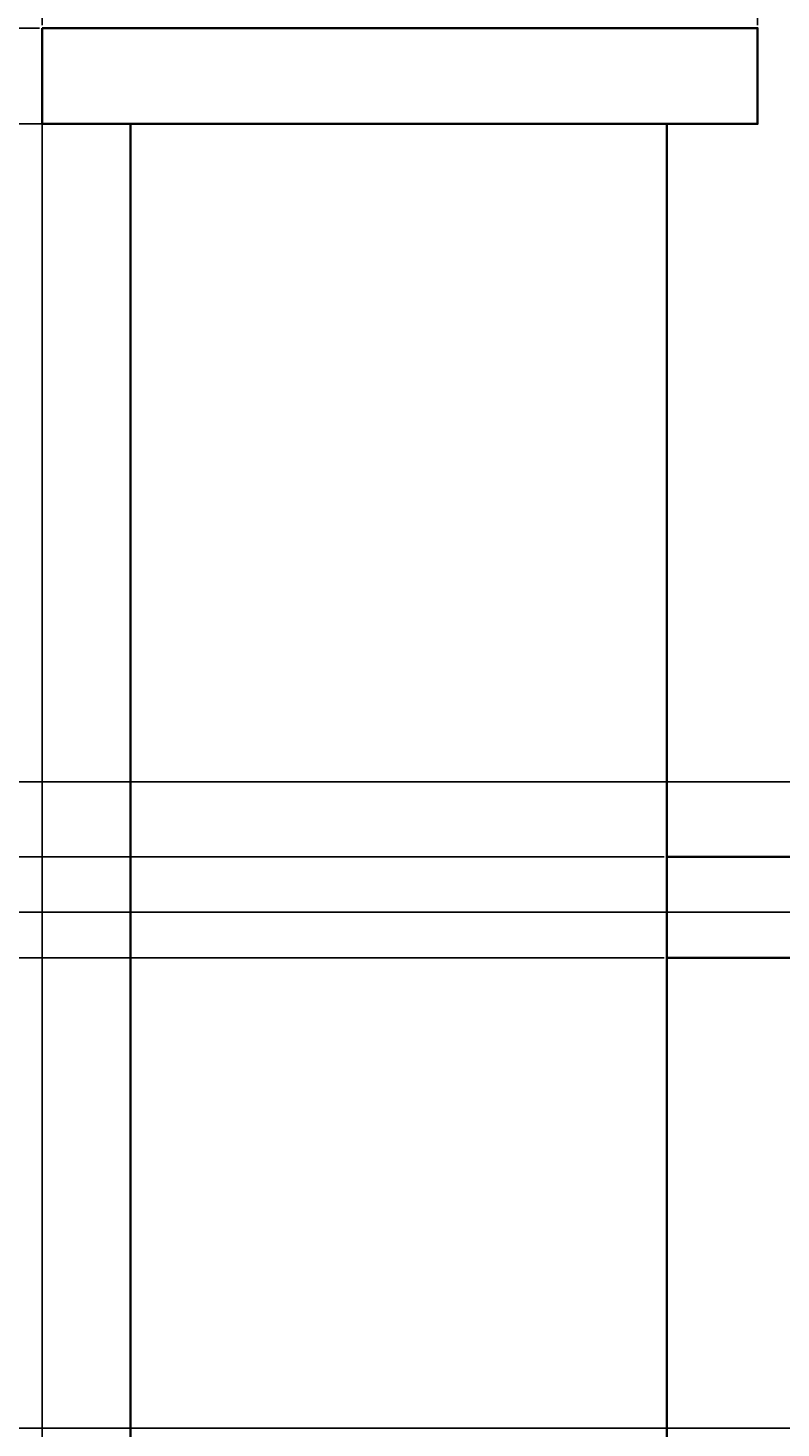
# Model space of a CAD drawing. Units: inches. Extents: x -6 to 289, y -8 to 323.
# Tile 6 of 107: x 10 to 27, y 36 to 68. Entities that reach past the tile are written whole.
import ezdxf

# ---------------------------------------------------------------- set-up
doc = ezdxf.new("R2010")
doc.units = ezdxf.units.IN
doc.header["$MEASUREMENT"] = 0
doc.layers.add('A-ANNO-DIMS', color=2, linetype='Continuous', lineweight=18)
doc.layers.add('A-ELEV', color=7, linetype='Continuous', lineweight=35)
doc.styles.get("Standard").update_dxf_attribs({"font": 'arial.ttf'})
doc.dimstyles.get("Standard").update_dxf_attribs({"dimtxt": 0.18, "dimasz": 0.18, "dimexe": 0.18, "dimexo": 0.0625, "dimgap": 0.09, "dimtad": 0, "dimtih": 1, "dimtoh": 1, "dimdec": 4, "dimzin": 0, "dimdsep": 46, "dimtxsty": 'Standard', "dimcen": 0.09, "dimadec": 0, "dimazin": 0, "dimtfac": 1, "dimtdec": 4, "dimtofl": 0, "dimtmove": 0, "dimatfit": 3, "dimfxl": 1, "dimtolj": 1, "dimtzin": 0, "dimarcsym": 0})

# ---------------------------------------------------------------- blocks, each defined once
blk = doc.blocks.new('*D16')
at = {"layer": 'A-ANNO-DIMS', "color": 0, "lineweight": -2, "transparency": 16777216}
for p, q in [((9.943, 68.37), (9.943, -8.391)), ((272.973, 68.37), (272.973, -8.391)), ((10.123, -8.211), (140.993, -8.211)), ((272.793, -8.211), (141.923, -8.211))]:
    blk.add_line(p, q, dxfattribs=at)
at = {"layer": 'A-ANNO-DIMS', "color": 0, "transparency": 16777216}
for points in [[(10.123, -8.181), (10.123, -8.241), (9.943, -8.211)], [(272.793, -8.181), (272.793, -8.241), (272.973, -8.211)]]:
    blk.add_solid(points, dxfattribs=at)
at = {"layer": 'Defpoints', "color": 0, "transparency": 16777216}
for p in [(9.943, 68.432), (272.973, 68.432), (272.973, -8.211)]:
    blk.add_point(p, dxfattribs=at)
at = {"layer": 'A-ANNO-DIMS', "color": 0, "transparency": 16777216, "insert": (141.458, -8.211), "char_height": 0.18, "attachment_point": 5}
blk.add_mtext('\\A1;263.03', dxfattribs=at)
blk = doc.blocks.new('*D17')
at = {"layer": 'A-ANNO-DIMS', "color": 0, "lineweight": -2, "transparency": 16777216}
for p, q in [((33.681, 70.243), (-5.737, 70.243)), ((-5.557, 70.063), (-5.557, 38.948)), ((-5.557, 7.469), (-5.557, 38.584)), ((11.907, 7.289), (-5.737, 7.289))]:
    blk.add_line(p, q, dxfattribs=at)
at = {"layer": 'A-ANNO-DIMS', "color": 0, "transparency": 16777216}
for points in [[(-5.587, 70.063), (-5.527, 70.063), (-5.557, 70.243)], [(-5.587, 7.469), (-5.527, 7.469), (-5.557, 7.289)]]:
    blk.add_solid(points, dxfattribs=at)
at = {"layer": 'Defpoints', "color": 0, "transparency": 16777216}
for p in [(-5.557, 70.243), (33.744, 70.243), (11.969, 7.289)]:
    blk.add_point(p, dxfattribs=at)
at = {"layer": 'A-ANNO-DIMS', "color": 0, "transparency": 16777216, "insert": (-5.557, 38.766), "char_height": 0.18, "attachment_point": 5}
blk.add_mtext('\\A1;62.95', dxfattribs=at)
blk = doc.blocks.new('*D22')
at = {"layer": 'A-ANNO-DIMS', "color": 0, "lineweight": -2, "transparency": 16777216}
for p, q in [((19.101, 307.289), (-5.737, 307.289)), ((-5.557, 307.109), (-5.557, 157.471)), ((-5.557, 7.469), (-5.557, 157.107)), ((11.907, 7.289), (-5.737, 7.289))]:
    blk.add_line(p, q, dxfattribs=at)
at = {"layer": 'A-ANNO-DIMS', "color": 0, "transparency": 16777216}
for points in [[(-5.587, 307.109), (-5.527, 307.109), (-5.557, 307.289)], [(-5.587, 7.469), (-5.527, 7.469), (-5.557, 7.289)]]:
    blk.add_solid(points, dxfattribs=at)
at = {"layer": 'Defpoints', "color": 0, "transparency": 16777216}
for p in [(19.164, 307.289), (-5.557, 7.289), (11.969, 7.289)]:
    blk.add_point(p, dxfattribs=at)
at = {"layer": 'A-ANNO-DIMS', "color": 0, "transparency": 16777216, "insert": (-5.557, 157.289), "char_height": 0.18, "attachment_point": 5}
blk.add_mtext('\\A1;300', dxfattribs=at)
blk = doc.blocks.new('*D57')
at = {"layer": 'A-ANNO-DIMS', "color": 0, "lineweight": -2, "transparency": 16777216}
for p, q in [((9.943, 68.495), (9.943, 322.969)), ((26.403, 68.495), (26.403, 322.969)), ((10.123, 322.789), (17.788, 322.789)), ((26.223, 322.789), (18.558, 322.789))]:
    blk.add_line(p, q, dxfattribs=at)
at = {"layer": 'A-ANNO-DIMS', "color": 0, "transparency": 16777216}
for points in [[(10.123, 322.819), (10.123, 322.759), (9.943, 322.789)], [(26.223, 322.819), (26.223, 322.759), (26.403, 322.789)]]:
    blk.add_solid(points, dxfattribs=at)
at = {"layer": 'Defpoints', "color": 0, "transparency": 16777216}
for p in [(26.403, 322.789), (9.943, 68.432), (26.403, 68.432)]:
    blk.add_point(p, dxfattribs=at)
at = {"layer": 'A-ANNO-DIMS', "color": 0, "transparency": 16777216, "insert": (18.173, 322.789), "char_height": 0.18, "attachment_point": 5}
blk.add_mtext('\\A1;16.46', dxfattribs=at)
blk = doc.blocks.new('*D62')
at = {"layer": 'A-ANNO-DIMS', "color": 0, "lineweight": -2, "transparency": 16777216}
for p, q in [((39.647, 36.213), (-5.737, 36.213)), ((-5.557, 36.033), (-5.557, 33.895)), ((-5.557, 31.393), (-5.557, 33.532)), ((44.647, 31.213), (-5.737, 31.213))]:
    blk.add_line(p, q, dxfattribs=at)
at = {"layer": 'A-ANNO-DIMS', "color": 0, "transparency": 16777216}
for points in [[(-5.587, 36.033), (-5.527, 36.033), (-5.557, 36.213)], [(-5.587, 31.393), (-5.527, 31.393), (-5.557, 31.213)]]:
    blk.add_solid(points, dxfattribs=at)
at = {"layer": 'Defpoints', "color": 0, "transparency": 16777216}
for p in [(-5.557, 36.213), (39.709, 36.213), (44.709, 31.213)]:
    blk.add_point(p, dxfattribs=at)
at = {"layer": 'A-ANNO-DIMS', "color": 0, "transparency": 16777216, "insert": (-5.557, 33.713), "char_height": 0.18, "attachment_point": 5}
blk.add_mtext('\\A1;5', dxfattribs=at)
blk = doc.blocks.new('*D63')
at = {"layer": 'A-ANNO-DIMS', "color": 0, "lineweight": -2, "transparency": 16777216}
for p, q in [((24.254, 47.03), (-5.737, 47.03)), ((-5.557, 46.85), (-5.557, 41.804)), ((-5.557, 36.393), (-5.557, 41.44)), ((39.647, 36.213), (-5.737, 36.213))]:
    blk.add_line(p, q, dxfattribs=at)
at = {"layer": 'A-ANNO-DIMS', "color": 0, "transparency": 16777216}
for points in [[(-5.587, 46.85), (-5.527, 46.85), (-5.557, 47.03)], [(-5.587, 36.393), (-5.527, 36.393), (-5.557, 36.213)]]:
    blk.add_solid(points, dxfattribs=at)
at = {"layer": 'Defpoints', "color": 0, "transparency": 16777216}
for p in [(-5.557, 47.03), (24.317, 47.03), (39.709, 36.213)]:
    blk.add_point(p, dxfattribs=at)
at = {"layer": 'A-ANNO-DIMS', "color": 0, "transparency": 16777216, "insert": (-5.557, 41.622), "char_height": 0.18, "attachment_point": 5}
blk.add_mtext('\\A1;10.817', dxfattribs=at)
blk = doc.blocks.new('*D64')
at = {"layer": 'A-ANNO-DIMS', "color": 0, "lineweight": -2, "transparency": 16777216}
for p, q in [((24.254, 49.36), (-5.737, 49.36)), ((-5.557, 49.18), (-5.557, 48.377)), ((-5.557, 47.21), (-5.557, 48.013)), ((24.254, 47.03), (-5.737, 47.03))]:
    blk.add_line(p, q, dxfattribs=at)
at = {"layer": 'A-ANNO-DIMS', "color": 0, "transparency": 16777216}
for points in [[(-5.587, 49.18), (-5.527, 49.18), (-5.557, 49.36)], [(-5.587, 47.21), (-5.527, 47.21), (-5.557, 47.03)]]:
    blk.add_solid(points, dxfattribs=at)
at = {"layer": 'Defpoints', "color": 0, "transparency": 16777216}
for p in [(-5.557, 49.36), (24.317, 49.36), (24.317, 47.03)]:
    blk.add_point(p, dxfattribs=at)
at = {"layer": 'A-ANNO-DIMS', "color": 0, "transparency": 16777216, "insert": (-5.557, 48.195), "char_height": 0.18, "attachment_point": 5}
blk.add_mtext('\\A1;2.33', dxfattribs=at)
blk = doc.blocks.new('*D65')
at = {"layer": 'A-ANNO-DIMS', "color": 0, "lineweight": -2, "transparency": 16777216}
for p, q in [((11.907, 66.224), (-5.737, 66.224)), ((-5.557, 66.044), (-5.557, 57.974)), ((-5.557, 49.54), (-5.557, 57.61)), ((24.254, 49.36), (-5.737, 49.36))]:
    blk.add_line(p, q, dxfattribs=at)
at = {"layer": 'A-ANNO-DIMS', "color": 0, "transparency": 16777216}
for points in [[(-5.587, 66.044), (-5.527, 66.044), (-5.557, 66.224)], [(-5.587, 49.54), (-5.527, 49.54), (-5.557, 49.36)]]:
    blk.add_solid(points, dxfattribs=at)
at = {"layer": 'Defpoints', "color": 0, "transparency": 16777216}
for p in [(-5.557, 66.224), (11.969, 66.224), (24.317, 49.36)]:
    blk.add_point(p, dxfattribs=at)
at = {"layer": 'A-ANNO-DIMS', "color": 0, "transparency": 16777216, "insert": (-5.557, 57.792), "char_height": 0.18, "attachment_point": 5}
blk.add_mtext('\\A1;16.863', dxfattribs=at)
blk = doc.blocks.new('*D66')
at = {"layer": 'A-ANNO-DIMS', "color": 0, "lineweight": -2, "transparency": 16777216}
for p, q in [((9.881, 68.432), (-5.737, 68.432)), ((-5.557, 68.252), (-5.557, 67.508)), ((-5.557, 66.404), (-5.557, 67.148)), ((11.907, 66.224), (-5.737, 66.224))]:
    blk.add_line(p, q, dxfattribs=at)
at = {"layer": 'A-ANNO-DIMS', "color": 0, "transparency": 16777216}
for points in [[(-5.587, 68.252), (-5.527, 68.252), (-5.557, 68.432)], [(-5.587, 66.404), (-5.527, 66.404), (-5.557, 66.224)]]:
    blk.add_solid(points, dxfattribs=at)
at = {"layer": 'Defpoints', "color": 0, "transparency": 16777216}
for p in [(-5.557, 68.432), (9.943, 68.432), (11.969, 66.224)]:
    blk.add_point(p, dxfattribs=at)
at = {"layer": 'A-ANNO-DIMS', "color": 0, "transparency": 16777216, "insert": (-5.557, 67.328), "char_height": 0.18, "attachment_point": 5}
blk.add_mtext('\\A1;2.21', dxfattribs=at)
blk = doc.blocks.new('*D84')
at = {"layer": 'A-ANNO-DIMS', "color": 0, "lineweight": -2, "transparency": 16777216}
for p, q in [((123.945, 48.085), (-5.737, 48.085)), ((-5.557, 47.905), (-5.557, 29.369)), ((-5.557, 10.469), (-5.557, 29.005)), ((123.945, 10.289), (-5.737, 10.289))]:
    blk.add_line(p, q, dxfattribs=at)
at = {"layer": 'A-ANNO-DIMS', "color": 0, "transparency": 16777216}
for points in [[(-5.587, 47.905), (-5.527, 47.905), (-5.557, 48.085)], [(-5.587, 10.469), (-5.527, 10.469), (-5.557, 10.289)]]:
    blk.add_solid(points, dxfattribs=at)
at = {"layer": 'Defpoints', "color": 0, "transparency": 16777216}
for p in [(-5.557, 48.085), (124.008, 48.085), (124.008, 10.289)]:
    blk.add_point(p, dxfattribs=at)
at = {"layer": 'A-ANNO-DIMS', "color": 0, "transparency": 16777216, "insert": (-5.557, 29.187), "char_height": 0.18, "attachment_point": 5}
blk.add_mtext('\\A1;37.8', dxfattribs=at)
blk = doc.blocks.new('*D85')
at = {"layer": 'A-ANNO-DIMS', "color": 0, "lineweight": -2, "transparency": 16777216}
for p, q in [((120.945, 51.085), (-5.737, 51.085)), ((-5.557, 50.905), (-5.557, 49.767)), ((-5.557, 48.265), (-5.557, 49.403)), ((123.945, 48.085), (-5.737, 48.085))]:
    blk.add_line(p, q, dxfattribs=at)
at = {"layer": 'A-ANNO-DIMS', "color": 0, "transparency": 16777216}
for points in [[(-5.587, 50.905), (-5.527, 50.905), (-5.557, 51.085)], [(-5.587, 48.265), (-5.527, 48.265), (-5.557, 48.085)]]:
    blk.add_solid(points, dxfattribs=at)
at = {"layer": 'Defpoints', "color": 0, "transparency": 16777216}
for p in [(-5.557, 51.085), (121.008, 51.085), (124.008, 48.085)]:
    blk.add_point(p, dxfattribs=at)
at = {"layer": 'A-ANNO-DIMS', "color": 0, "transparency": 16777216, "insert": (-5.557, 49.585), "char_height": 0.18, "attachment_point": 5}
blk.add_mtext('\\A1;3', dxfattribs=at)
blk = doc.blocks.new('*D86')
at = {"layer": 'A-ANNO-DIMS', "color": 0, "lineweight": -2, "transparency": 16777216}
for p, q in [((166.233, 75.971), (-5.737, 75.971)), ((-5.557, 75.791), (-5.557, 63.71)), ((-5.557, 51.265), (-5.557, 63.346)), ((120.945, 51.085), (-5.737, 51.085))]:
    blk.add_line(p, q, dxfattribs=at)
at = {"layer": 'A-ANNO-DIMS', "color": 0, "transparency": 16777216}
for points in [[(-5.587, 75.791), (-5.527, 75.791), (-5.557, 75.971)], [(-5.587, 51.265), (-5.527, 51.265), (-5.557, 51.085)]]:
    blk.add_solid(points, dxfattribs=at)
at = {"layer": 'Defpoints', "color": 0, "transparency": 16777216}
for p in [(-5.557, 75.971), (166.296, 75.971), (121.008, 51.085)]:
    blk.add_point(p, dxfattribs=at)
at = {"layer": 'A-ANNO-DIMS', "color": 0, "transparency": 16777216, "insert": (-5.557, 63.528), "char_height": 0.18, "attachment_point": 5}
blk.add_mtext('\\A1;24.886', dxfattribs=at)

msp = doc.modelspace()

# ---------------------------------------------------------------- linework, layer by layer
at = {"layer": 'A-ELEV'}
for points in [[(9.943, 68.4322), (26.403, 68.4322), (26.403, 66.2238), (9.943, 66.2238)], [(24.317, 49.3604), (108.6602, 49.3604), (108.6602, 7.2888), (24.317, 7.2888)], [(24.317, 49.3604), (108.6602, 49.3604), (108.6602, 47.0304), (24.317, 47.0304)]]:
    msp.add_lwpolyline(points, close=True, dxfattribs=at)
msp.add_lwpolyline([(11.9692, 66.2238), (11.9692, 7.2888), (24.317, 7.2888), (24.317, 66.2238)], dxfattribs=at)

# ---------------------------------------------------------------- dimensions: what is measured, and where the dimension line sits
at = {"layer": 'A-ANNO-DIMS'}
for base, p2, picture, middle in [((26.403, 322.7888), (26.403, 68.4322), '*D57', (18.173, 322.7888)), ((272.9733, -8.2112), (272.9733, 68.4322), '*D16', (141.4581, -8.2112))]:
    dim = msp.add_linear_dim(base=base, p1=(9.943, 68.4322), p2=p2, dimstyle='Standard', override={"dimdec": 2, "dimlfac": 1, "dimrnd": 0, "dimzin": 0, "dimdsep": 46, "dimlunit": 2}, dxfattribs=at)
    dim.commit()
    dim.dimension.update_dxf_attribs({"geometry": picture, "text_midpoint": middle})
for base, p1, p2, override, picture, middle in [((-5.557, 7.2888), (19.1638, 307.2888), (11.9692, 7.2888), {"dimdec": 0, "dimlfac": 1, "dimrnd": 0, "dimzin": 0, "dimdsep": 46, "dimlunit": 2}, '*D22', (-5.557, 157.2888)), ((-5.557, 75.97064), (121.00798, 51.08513), (166.29599, 75.97064), {"dimdec": 3, "dimlfac": 1, "dimrnd": 0, "dimzin": 0, "dimdsep": 46, "dimlunit": 2}, '*D86', (-5.557, 63.52788)), ((-5.557, 70.2425), (11.9692, 7.2888), (33.7437, 70.2425), {"dimdec": 2, "dimlfac": 1, "dimrnd": 0, "dimzin": 0, "dimdsep": 46, "dimlunit": 2}, '*D17', (-5.557, 38.7657)), ((-5.557, 68.4322), (11.9692, 66.2238), (9.943, 68.4322), {"dimdec": 2, "dimlfac": 1, "dimrnd": 0, "dimzin": 0, "dimdsep": 46, "dimlunit": 2}, '*D66', (-5.557, 67.328)), ((-5.557, 66.2238), (24.317, 49.3604), (11.9692, 66.2238), {"dimdec": 3, "dimlfac": 1, "dimrnd": 0, "dimzin": 0, "dimdsep": 46, "dimlunit": 2}, '*D65', (-5.557, 57.7921)), ((-5.557, 51.0851), (124.008, 48.0851), (121.008, 51.0851), {"dimdec": 0, "dimlfac": 1, "dimrnd": 0, "dimzin": 0, "dimdsep": 46, "dimlunit": 2}, '*D85', (-5.557, 49.5851)), ((-5.557, 49.3604), (24.317, 47.0304), (24.317, 49.3604), {"dimdec": 2, "dimlfac": 1, "dimrnd": 0, "dimzin": 0, "dimdsep": 46, "dimlunit": 2}, '*D64', (-5.557, 48.1954)), ((-5.557, 48.0851), (124.008, 10.2888), (124.008, 48.0851), {"dimdec": 1, "dimlfac": 1, "dimrnd": 0, "dimzin": 0, "dimdsep": 46, "dimlunit": 2}, '*D84', (-5.557, 29.187)), ((-5.557, 47.0304), (39.709, 36.2133), (24.317, 47.0304), {"dimdec": 3, "dimlfac": 1, "dimrnd": 0, "dimzin": 0, "dimdsep": 46, "dimlunit": 2}, '*D63', (-5.557, 41.6219)), ((-5.557, 36.2133), (44.709, 31.2133), (39.709, 36.2133), {"dimdec": 0, "dimlfac": 1, "dimrnd": 0, "dimzin": 0, "dimdsep": 46, "dimlunit": 2}, '*D62', (-5.557, 33.7133))]:
    dim = msp.add_linear_dim(base=base, p1=p1, p2=p2, angle=90, dimstyle='Standard', override=override, dxfattribs=at)
    dim.commit()
    dim.dimension.update_dxf_attribs({"geometry": picture, "text_midpoint": middle})

doc.saveas('drawing.dxf')
